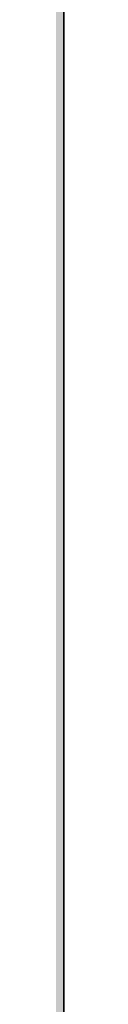
# Model space of a CAD drawing. Units: inches. Extents: x 2091 to 2899, y 967 to 2217.
# Tile 68 of 256: x 2212.144 to 2212.144, y 1101.165 to 1102.499. Entities that reach past the tile are written whole.
import ezdxf

# ---------------------------------------------------------------- set-up
doc = ezdxf.new("R2010")
doc.units = ezdxf.units.IN
doc.layers.add('A-WALL', color=7, linetype='Continuous', lineweight=35)
doc.layers.add('A-WALL-PATT', color=141, linetype='Continuous', lineweight=13, true_color=0xadddf7)

msp = doc.modelspace()

# ---------------------------------------------------------------- hatches: boundary and pattern name
at = {"layer": 'A-WALL-PATT'}
h = msp.add_hatch(color=256, dxfattribs=at)
h.dxf.hatch_style = 1
h.paths.add_polyline_path([(2212.1436, 1941.4191), (2387.6436, 1941.4191), (2387.6436, 1824.4191), (2392.1436, 1824.4191), (2392.1436, 1941.4191), (2609.6436, 1941.4191), (2609.6436, 1825.9191), (2614.1436, 1825.9191), (2614.1436, 1941.4191), (2794.1436, 1941.4191), (2794.1436, 1928.7622), (2803.1436, 1928.7622), (2803.1436, 2050.9191), (2203.1436, 2050.9191), (2203.1436, 1900.7579), (2212.1436, 1900.7579)])
h.paths.add_polyline_path([(2212.1436, 1945.9191), (2212.1436, 2041.9191), (2794.1436, 2041.9191), (2794.1436, 1945.9191), (2402.2482, 1945.9191), (2401.1024, 1945.7758), (2398.7024, 1945.7758)], flags=16)
h.paths.add_polyline_path([(2230.2299, 1948.0628), (2227.3499, 1949.5028), (2225.9099, 1951.9028), (2223.9899, 1952.8628), (2223.0299, 1955.2628), (2222.0699, 1959.5828), (2222.0699, 1963.4228), (2223.0299, 1965.6628), (2223.9899, 1965.3428), (2225.5859, 1963.8607), (2226.9115, 1964.9573), (2226.9489, 1965.9388), (2227.7783, 1966.9521), (2228.1999, 1968.8787), (2230.7099, 1964.8628), (2233.5899, 1966.3028), (2233.6073, 1966.3319), (2233.7727, 1964.9382), (2234.6338, 1963.6765), (2235.0299, 1963.9028), (2236.282, 1965.5724), (2235.9899, 1962.9428), (2237.9545, 1957.54), (2238.3899, 1957.9028), (2239.2159, 1960.3058), (2238.6546, 1966.385), (2238.6928, 1966.4381), (2238.8406, 1967.4997), (2238.7803, 1967.6875), (2238.8805, 1967.7868), (2238.6669, 1966.2518), (2239.2159, 1960.3058), (2238.3899, 1957.9028), (2236.9499, 1956.7028), (2234.5499, 1949.9828)], flags=0)
h.paths.add_polyline_path([(2278.012, 1948.0628), (2276.4964, 1947.8733), (2275.8498, 1947.6886), (2274.652, 1947.1028)], flags=0)
h.paths.add_polyline_path([(2269.852, 1955.7428), (2268.2762, 1956.6293), (2270.8673, 1956.3484), (2269.372, 1958.1428), (2268.715, 1959.1923), (2270.5698, 1958.7286), (2268.5807, 1961.9061), (2270.812, 1960.8919), (2270.812, 1963.4228), (2271.3933, 1964.7793), (2270.2918, 1966.1562), (2271.772, 1965.6628), (2272.1414, 1966.5248), (2273.9298, 1965.9286), (2275.6304, 1968.0543), (2276.3319, 1966.7219), (2276.5204, 1966.9521), (2276.942, 1968.8787), (2277.7343, 1967.6111), (2278.1399, 1969.4645), (2279.6591, 1967.0337), (2280.412, 1966.7828), (2280.9493, 1967.5888), (2281.6098, 1967.3686), (2282.1333, 1968.1538), (2282.3492, 1966.3334), (2282.3498, 1966.3326), (2283.4076, 1968.0954), (2283.7126, 1965.524), (2284.3202, 1964.6338), (2284.5118, 1964.8892), (2284.235, 1965.7048), (2284.5005, 1967.319), (2284.9079, 1965.4174), (2285.3963, 1966.0686), (2285.4328, 1966.2906), (2285.4733, 1966.1713), (2286.3539, 1967.3454), (2286.222, 1966.1582), (2287.6635, 1968.0802), (2287.714, 1968.4428), (2288.4816, 1969.0167), (2288.574, 1968.7289), (2288.9175, 1969.069), (2288.6068, 1966.8376), (2288.9287, 1963.3513), (2288.935, 1963.3568), (2288.9297, 1963.3404), (2289.0153, 1962.4139), (2290.1112, 1963.8751), (2290.1328, 1963.9426), (2290.2177, 1964.0171), (2290.1112, 1963.8751), (2289.1558, 1960.8916), (2288.594, 1959.2572), (2288.572, 1959.1028), (2289.532, 1960.5428), (2290.012, 1962.4628), (2290.1918, 1962.6427), (2289.7698, 1959.6886), (2286.8898, 1957.2886), (2284.4898, 1950.5686), (2283.3147, 1950.0463), (2283.292, 1949.9828), (2280.2901, 1948.6486), (2281.1298, 1948.6486), (2282.5698, 1948.1686), (2283.2047, 1948.0628), (2278.972, 1948.0628), (2276.092, 1949.5028), (2274.652, 1951.9028), (2272.732, 1952.8628)], flags=0)
h.paths.add_polyline_path([(2271.1589, 1958.0218), (2272.9698, 1955.8486), (2272.0098, 1960.1686), (2272.0098, 1964.0086), (2272.6244, 1965.4427), (2274.328, 1963.8607), (2275.6536, 1964.9573), (2275.6377, 1964.5391), (2277.4122, 1966.0069), (2277.033, 1965.1568), (2276.8299, 1964.9756), (2276.766, 1963.295), (2277.4496, 1962.6602), (2279.452, 1964.8628), (2282.332, 1966.3028), (2283.5298, 1966.8886), (2283.2945, 1966.7709), (2283.913, 1963.8847), (2284.8992, 1964.4483), (2284.732, 1962.9428), (2286.6966, 1957.54), (2287.132, 1957.9028), (2287.5419, 1959.0954), (2287.7794, 1958.4423), (2285.6827, 1956.6951), (2285.8765, 1959.7953), (2284.732, 1962.9428), (2284.8992, 1964.4483), (2283.913, 1963.8847), (2284.2238, 1962.4341), (2283.4244, 1963.6055), (2281.6098, 1962.5686), (2281.1298, 1960.1686), (2282.0898, 1956.3286), (2283.0498, 1952.9686), (2282.5698, 1950.5686), (2280.1698, 1948.6486), (2279.8833, 1948.7919), (2278.972, 1948.0628), (2278.972, 1949.0228), (2278.6723, 1949.3974), (2277.2898, 1950.0886), (2275.8498, 1952.4886), (2273.9298, 1953.4486), (2272.4898, 1954.8886), (2271.9216, 1954.8886), (2271.772, 1955.2628)], flags=0)
h.paths.add_polyline_path([(2311.9941, 1955.7428), (2312.0627, 1955.6742), (2312.0551, 1955.7085)], flags=0)
h.paths.add_polyline_path([(2331.9561, 1963.9518), (2333.3961, 1965.3918), (2331.0771, 1963.3568), (2330.9986, 1963.1115)], flags=0)
h.paths.add_polyline_path([(2310.5541, 1954.3028), (2307.0398, 1956.2799), (2310.7629, 1955.8763), (2312.4741, 1953.8228), (2313.4341, 1951.4228), (2315.3541, 1950.4628), (2316.7941, 1948.0628), (2317.4661, 1947.7268), (2319.3687, 1947.9646), (2317.7541, 1949.9828), (2317.5695, 1950.6105), (2316.7941, 1951.9028), (2314.8741, 1952.8628), (2313.9141, 1955.2628), (2311.5141, 1958.1428), (2309.3755, 1961.5592), (2311.5141, 1960.3371), (2311.5141, 1961.9828), (2310.6047, 1963.1196), (2311.7266, 1962.4785), (2312.4183, 1964.0926), (2312.256, 1964.2955), (2313.1941, 1963.9828), (2313.9141, 1965.6628), (2314.6468, 1965.4186), (2315.3541, 1966.3028), (2316.7941, 1967.7428), (2316.1574, 1966.9469), (2317.0341, 1965.2819), (2317.2226, 1965.5121), (2317.777, 1968.0458), (2318.4741, 1966.7219), (2318.6626, 1966.9521), (2319.0842, 1968.8787), (2321.207, 1965.4821), (2322.1614, 1966.9137), (2322.5541, 1966.7828), (2322.786, 1967.1306), (2322.8816, 1966.3243), (2323.312, 1965.7217), (2323.6513, 1965.8914), (2324.3965, 1967.1334), (2324.6569, 1964.9382), (2324.972, 1964.4766), (2325.3873, 1967.0015), (2325.9408, 1964.4183), (2327.2289, 1966.1358), (2327.1663, 1965.5724), (2328.0591, 1966.7628), (2328.2246, 1966.2475), (2329.668, 1967.6769), (2329.6646, 1967.6875), (2329.7648, 1967.7868), (2329.5511, 1966.2518), (2330.1001, 1960.3058), (2329.3328, 1958.0735), (2329.3131, 1957.9352), (2329.6341, 1958.2028), (2330.2341, 1959.1028), (2330.7141, 1961.0228), (2331.0341, 1961.3428), (2330.7141, 1959.1028), (2329.6341, 1958.2028), (2329.2741, 1957.6628), (2327.7121, 1956.3611), (2325.4341, 1949.9828), (2324.3338, 1949.4937), (2323.9941, 1948.5428), (2319.6741, 1946.6228), (2316.7941, 1948.0628), (2315.3541, 1950.4628), (2313.4341, 1951.4228)], flags=0)
h.paths.add_polyline_path([(2321.3357, 1947.952), (2321.1141, 1948.0628), (2321.1141, 1949.0228), (2319.1941, 1951.4228), (2316.7941, 1959.5828), (2316.6632, 1959.5828), (2315.3541, 1958.1428), (2314.3941, 1958.1428), (2313.1483, 1958.7091), (2312.9541, 1959.5828), (2312.9541, 1960.8919), (2315.8341, 1959.5828), (2316.6632, 1959.5828), (2317.3147, 1960.2994), (2315.0302, 1962.4207), (2316.3558, 1963.5173), (2316.3723, 1963.9516), (2316.4702, 1963.8607), (2317.7958, 1964.9573), (2317.7552, 1963.8897), (2319.1751, 1965.1568), (2319.4984, 1965.8814), (2321.1141, 1965.3428), (2323.2359, 1962.3724), (2325.6863, 1963.7726), (2325.5428, 1962.4806), (2325.1988, 1963.494), (2324.4785, 1963.0824), (2324.926, 1960.9941), (2324.0781, 1962.2365), (2322.4148, 1961.286), (2322.0741, 1959.5828), (2323.0341, 1955.7428), (2323.9941, 1952.3828), (2323.5141, 1949.9828), (2322.1427, 1948.8856), (2322.0741, 1948.5428)], flags=0)
h.paths.add_polyline_path([(2320.2075, 1963.3375), (2320.1541, 1963.4228), (2320.3941, 1963.5428)], flags=0)
h.paths.add_polyline_path([(2353.8505, 1965.8105), (2354.0305, 1965.7505), (2354.3305, 1966.4505), (2354.3305, 1966.9305)], flags=0)
h.paths.add_polyline_path([(2359.0206, 1969.0264), (2359.0984, 1968.9019), (2359.2335, 1969.5195), (2359.2335, 1969.9995)], flags=0)
h.paths.add_polyline_path([(2358.2567, 1966.6817), (2357.9836, 1966.348), (2358.2113, 1966.1462), (2358.4105, 1966.3896)], flags=0)
h.paths.add_polyline_path([(2357.7685, 1966.0588), (2357.7322, 1965.105), (2357.751, 1965.1206), (2357.7695, 1965.6065), (2357.7695, 1966.0578)], flags=0)
h.paths.add_polyline_path([(2359.1115, 1965.3045), (2359.1115, 1964.8245), (2359.8445, 1966.4675), (2359.8445, 1966.9475)], flags=0)
h.paths.add_polyline_path([(2360.2237, 1966.6214), (2360.6985, 1969.3625), (2360.6985, 1969.8425), (2360.2105, 1967.0255), (2360.2105, 1966.6425)], flags=0)
h.paths.add_polyline_path([(2363.4505, 1967.8905), (2363.4505, 1968.3705), (2362.4905, 1966.9305), (2362.656, 1966.6988)], flags=0)
h.paths.add_polyline_path([(2364.4755, 1966.0788), (2365.8505, 1968.3705), (2365.8505, 1968.8505), (2364.428, 1966.4796)], flags=0)
h.paths.add_polyline_path([(2366.3135, 1965.8525), (2366.3667, 1965.6958), (2366.8025, 1968.3455), (2366.8025, 1968.8255)], flags=0)
h.paths.add_polyline_path([(2367.1653, 1965.8035), (2367.2905, 1966.9305), (2367.2905, 1967.4105), (2367.1027, 1965.7201)], flags=0)
h.paths.add_polyline_path([(2370.0365, 1959.9735), (2371.0135, 1963.0245), (2371.0135, 1963.5045), (2370.0365, 1960.4535)], flags=0)
h.paths.add_polyline_path([(2371.6105, 1960.2105), (2372.5705, 1961.6505), (2372.5705, 1962.1305), (2371.8025, 1960.9785)], flags=0)
h.paths.add_polyline_path([(2350.8737, 1956.0051), (2351.9305, 1955.8905), (2354.4905, 1953.3305), (2353.8505, 1954.9305), (2351.4505, 1957.8105), (2347.9355, 1963.4255), (2347.9355, 1963.9055), (2351.4505, 1958.2905), (2353.7051, 1955.585), (2352.8905, 1959.2505), (2352.8905, 1959.7305), (2352.8905, 1961.9248), (2356.7305, 1959.7305), (2358.4545, 1961.6268), (2354.8105, 1965.0105), (2355.0309, 1965.2859), (2358.6911, 1961.8871), (2361.5305, 1965.0105), (2364.3765, 1966.4335), (2364.5244, 1965.1869), (2365.4545, 1963.8242), (2365.8811, 1964.068), (2365.3705, 1966.4505), (2365.3705, 1966.9305), (2366.8105, 1960.2105), (2366.8105, 1959.7305), (2366.3887, 1952.9814), (2367.7705, 1956.8505), (2368.6412, 1957.5761), (2366.8105, 1962.6105), (2366.8105, 1963.0905), (2368.7752, 1957.6877), (2369.2105, 1958.0505), (2370.0016, 1960.3519), (2369.4752, 1966.0527), (2369.5135, 1966.1058), (2369.5142, 1966.1109), (2369.4752, 1966.5327), (2369.5135, 1966.5858), (2369.6146, 1967.3126), (2369.1825, 1968.6585), (2369.1825, 1969.1385), (2369.601, 1967.8352), (2369.7012, 1967.9345), (2369.7179, 1968.0547), (2370.1452, 1968.3741), (2369.7787, 1968.0112), (2369.7012, 1967.4545), (2370.4682, 1968.214), (2369.6749, 1967.2658), (2369.5142, 1966.1109), (2370.0365, 1960.4535), (2370.0365, 1959.9735), (2369.4418, 1958.2432), (2370.6505, 1959.2505), (2371.0458, 1962.0176), (2371.1305, 1962.1305), (2370.6505, 1958.7705), (2367.7705, 1956.3705), (2365.3705, 1949.6505), (2362.0791, 1948.1876), (2363.4505, 1947.7305), (2361.0505, 1947.7305), (2360.0905, 1947.7305), (2357.1039, 1947.3572), (2360.0905, 1948.2105), (2358.1705, 1949.1705), (2356.7305, 1951.5705), (2354.8105, 1952.5305), (2351.9305, 1955.4105)], flags=0)
h.paths.add_polyline_path([(2361.0505, 1948.6905), (2359.1305, 1951.0905), (2356.7305, 1959.2505), (2355.7705, 1959.2505), (2352.8905, 1960.5596), (2352.8905, 1961.4448), (2355.8905, 1959.7305), (2356.7305, 1959.7305), (2356.8372, 1959.3678), (2361.5305, 1964.5305), (2363.2484, 1965.3894), (2364.9253, 1963.0418), (2362.4905, 1961.6505), (2362.0639, 1959.5172), (2362.9705, 1955.8905), (2363.9305, 1952.5305), (2363.9305, 1952.0505), (2363.4505, 1949.6505), (2361.0505, 1947.7305)], flags=0)
h.paths.add_polyline_path([(2359.1305, 1951.5705), (2359.2905, 1951.3705), (2361.0505, 1954.4505), (2361.0505, 1954.9305)], flags=0)
h.paths.add_polyline_path([(2357.2195, 1966.5455), (2356.7925, 1968.8145), (2356.7925, 1969.2945), (2357.2195, 1967.0255)], flags=0)
h.paths.add_polyline_path([(2361.0505, 1954.4505), (2361.5305, 1958.7705), (2361.5305, 1959.2505), (2361.0505, 1954.9305)], flags=0)
h.paths.add_polyline_path([(2402.5483, 1948.4861), (2402.3024, 1948.4158), (2402.5904, 1948.4158)], flags=0)
h.paths.add_polyline_path([(2394.1424, 1956.0958), (2395.6851, 1954.5532), (2396.7205, 1953.9707), (2396.0624, 1955.6158), (2395.2414, 1956.6011), (2395.8789, 1956.4417), (2395.1024, 1959.9358), (2395.1024, 1963.7758), (2396.0624, 1966.0158), (2397.0224, 1965.6958), (2398.6185, 1964.2138), (2399.9441, 1965.3103), (2399.9814, 1966.2918), (2400.8109, 1967.3052), (2401.2325, 1969.2317), (2403.5379, 1965.543), (2403.942, 1967.3893), (2404.7024, 1967.1358), (2405.4603, 1966.0748), (2406.6224, 1966.6558), (2406.6399, 1966.6849), (2406.8052, 1965.2912), (2406.9257, 1965.1147), (2407.3424, 1964.9758), (2407.8743, 1965.7737), (2408.1691, 1964.3981), (2409.3146, 1965.9254), (2409.2175, 1965.0511), (2409.4452, 1963.1312), (2410.3064, 1961.8695), (2410.7024, 1962.0958), (2411.4423, 1963.0823), (2411.1654, 1963.8978), (2411.6164, 1966.6398), (2411.7254, 1966.7911), (2411.8732, 1967.8527), (2411.8129, 1968.0405), (2411.9131, 1968.1398), (2411.6994, 1966.6048), (2412.2484, 1960.6588), (2413.2254, 1963.7098), (2414.3779, 1964.7212), (2414.5132, 1965.6927), (2414.4529, 1965.8805), (2414.5531, 1965.9798), (2414.3779, 1964.7212), (2414.5198, 1964.8457), (2414.3654, 1964.6311), (2414.3394, 1964.4448), (2414.8884, 1958.4988), (2414.0624, 1956.0958), (2412.6224, 1954.8958), (2410.1714, 1948.0329), (2410.0167, 1948.0844), (2405.9024, 1946.2558), (2405.9024, 1947.2158), (2405.2043, 1948.0886), (2404.2224, 1948.4158), (2403.2624, 1948.4158), (2400.3824, 1949.8558), (2399.6624, 1951.0558), (2397.9824, 1952.7358), (2397.0224, 1953.2158), (2395.6851, 1954.5532), (2392.6568, 1956.2569)], flags=0)
h.paths.add_polyline_path([(2409.0857, 1964.4074), (2409.1304, 1964.2757), (2409.2624, 1964.4958)], flags=0)
h.paths.add_polyline_path([(2397.7424, 1961.6158), (2398.7024, 1963.8558), (2399.6624, 1963.5358), (2401.4266, 1965.741), (2401.7914, 1966.5588), (2402.0714, 1965.0708), (2402.8355, 1964.3934), (2403.2624, 1964.9149), (2403.3381, 1964.7711), (2402.6155, 1963.9762), (2402.4986, 1960.9022), (2403.543, 1959.9325), (2404.4132, 1960.8897), (2404.7024, 1962.3358), (2407.9163, 1964.1724), (2409.5202, 1961.9269), (2410.9871, 1957.893), (2411.4224, 1958.2558), (2412.048, 1960.0756), (2412.4103, 1959.0791), (2411.6756, 1958.4668), (2411.6624, 1958.2558), (2411.6261, 1958.4255), (2409.9824, 1957.0558), (2407.5824, 1950.3358), (2403.2624, 1948.4158), (2403.2624, 1949.3758), (2401.3424, 1951.7758), (2399.4165, 1958.324), (2397.7424, 1959.0849), (2397.7424, 1959.9701), (2397.1024, 1960.3358), (2397.7424, 1960.0449)], flags=0)
h.paths.add_polyline_path([(2405.9024, 1952.9758), (2405.9504, 1953.4078), (2406.0167, 1953.1758)], flags=0)
h.paths.add_polyline_path([(2449.8178, 1967.114), (2449.7523, 1967.1358), (2449.7937, 1967.0779)], flags=0)
h.paths.add_polyline_path([(2451.6977, 1966.6181), (2451.7409, 1966.6901), (2451.6921, 1966.6657)], flags=0)
h.paths.add_polyline_path([(2454.3436, 1965.7376), (2455.7523, 1967.6158), (2455.9923, 1968.0958), (2454.3645, 1965.9254)], flags=0)
h.paths.add_polyline_path([(2457.5473, 1968.8638), (2457.7873, 1969.3438), (2457.0543, 1968.7958), (2457.0076, 1968.4603)], flags=0)
h.paths.add_polyline_path([(2456.9218, 1967.8567), (2456.8022, 1968.229), (2456.723, 1967.6598)], flags=0)
h.paths.add_polyline_path([(2457.3023, 1967.3768), (2457.5423, 1967.8568), (2456.8103, 1966.8398), (2456.7405, 1966.7002), (2456.749, 1966.6081)], flags=0)
h.paths.add_polyline_path([(2458.2753, 1963.7098), (2458.1553, 1963.3352), (2460.3543, 1965.2648), (2460.5943, 1965.7448)], flags=0)
h.paths.add_polyline_path([(2458.3923, 1962.8158), (2458.3641, 1962.6182), (2459.5923, 1964.2558), (2459.8323, 1964.7358)], flags=0)
h.paths.add_polyline_path([(2459.3523, 1962.8158), (2459.2723, 1962.4958), (2460.0723, 1963.2958), (2460.3123, 1963.7758)], flags=0)
h.paths.add_polyline_path([(2458.6803, 1960.6078), (2458.6323, 1960.4158), (2459.5923, 1961.8558), (2459.8323, 1962.3358)], flags=0)
h.paths.add_polyline_path([(2437.8382, 1956.2427), (2439.1923, 1956.0958), (2441.3523, 1953.9358), (2440.8723, 1955.1358), (2438.4723, 1958.0158), (2438.0716, 1958.656), (2438.7123, 1958.4958), (2440.6396, 1956.1831), (2439.9123, 1959.4558), (2439.9123, 1963.2958), (2441.3523, 1966.6558), (2441.5923, 1967.1358), (2441.1123, 1966.0158), (2442.0723, 1965.6958), (2443.989, 1968.0917), (2444.2413, 1966.7508), (2444.9168, 1966.1519), (2445.6766, 1967.0801), (2446.2553, 1969.7248), (2446.4953, 1970.2048), (2446.2824, 1969.2317), (2447.3627, 1967.5033), (2447.7203, 1969.5678), (2447.9603, 1970.0478), (2447.4855, 1967.3068), (2448.7923, 1965.2158), (2448.4723, 1964.8638), (2448.5523, 1964.7358), (2451.4521, 1966.1857), (2451.6151, 1964.8112), (2452.3079, 1963.7962), (2453.2345, 1964.3257), (2454.0723, 1960.4158), (2453.6287, 1953.3177), (2454.7923, 1956.5758), (2455.0323, 1957.0558), (2455.7188, 1957.6279), (2453.8323, 1962.8158), (2453.941, 1963.7936), (2453.3353, 1965.5778), (2453.8243, 1968.5508), (2454.0643, 1969.0308), (2453.5753, 1966.0578), (2454.0403, 1964.6879), (2453.8323, 1962.8158), (2455.7188, 1957.6279), (2456.3672, 1958.1682), (2457.0583, 1960.1788), (2457.2983, 1960.6588), (2456.4723, 1958.2558), (2457.7177, 1959.2937), (2457.6723, 1958.9758), (2454.89, 1956.6572), (2453.6141, 1953.0849), (2453.5923, 1952.7358), (2453.3523, 1952.2558), (2453.3596, 1952.3722), (2452.6323, 1950.3358), (2452.3923, 1949.8558), (2449.2038, 1948.4387), (2450.7123, 1947.9358), (2448.0723, 1947.9358), (2447.1123, 1947.9358), (2444.5523, 1947.6158), (2447.1996, 1948.3722), (2445.1923, 1949.3758), (2443.7523, 1951.7758), (2441.8323, 1952.7358), (2438.9523, 1955.6158)], flags=0)
h.paths.add_polyline_path([(2443.9923, 1959.9358), (2444.0403, 1959.7726), (2444.1216, 1959.862)], flags=0)
h.paths.add_polyline_path([(2442.9123, 1959.9358), (2443.0323, 1959.9358), (2442.4457, 1960.2025)], flags=0)
h.paths.add_polyline_path([(2444.9829, 1965.0197), (2445.2793, 1965.2648), (2445.5193, 1965.7448), (2444.994, 1965.3103)], flags=0)
h.paths.add_polyline_path([(2446.1333, 1965.0298), (2446.3304, 1965.4715), (2444.9703, 1964.2578), (2444.7303, 1963.7778)], flags=0)
h.paths.add_polyline_path([(2442.7923, 1959.4558), (2443.7523, 1959.4558), (2446.1523, 1951.2958), (2446.4123, 1951.7508), (2446.3923, 1951.7758), (2448.0806, 1954.7303), (2448.5523, 1958.9758), (2441.8323, 1965.2158), (2442.1549, 1965.6191), (2448.7923, 1959.4558), (2448.3123, 1955.1358), (2448.0723, 1954.6558), (2446.4123, 1951.7508), (2448.3123, 1949.3758), (2448.3123, 1948.4158), (2450.5409, 1950.1987), (2450.9523, 1952.2558), (2449.9923, 1955.6158), (2449.0323, 1959.4558), (2449.5123, 1961.8558), (2449.7523, 1962.3358), (2449.6749, 1961.9487), (2452.9945, 1963.8457), (2453.0644, 1963.5194), (2452.8846, 1963.7829), (2449.6749, 1961.9487), (2449.2723, 1959.9358), (2450.2323, 1956.0958), (2451.1923, 1952.7358), (2450.7123, 1950.3358), (2450.4723, 1949.8558), (2448.0723, 1947.9358), (2448.0723, 1948.5358), (2445.4323, 1949.8558), (2443.9923, 1952.2558), (2442.0723, 1953.2158), (2441.1123, 1955.6158), (2440.1523, 1959.9358), (2440.1523, 1960.6558)], flags=0)
h.paths.add_polyline_path([(2456.6923, 1966.9858), (2457.6083, 1968.0808), (2457.8483, 1968.5608), (2456.9323, 1967.4658)], flags=0)
h.paths.add_polyline_path([(2489.8966, 1966.5802), (2489.9429, 1966.1893), (2490.7475, 1967.5302), (2491.3191, 1968.9512)], flags=0)
h.paths.add_polyline_path([(2473.5625, 1956.4071), (2477.14, 1956.0193), (2476.9553, 1956.2408), (2475.108, 1957.2801), (2476.3475, 1956.9702), (2475.1869, 1958.8242), (2476.9191, 1958.3912), (2475.4116, 1960.7993), (2477.7875, 1959.7193), (2477.7875, 1962.2502), (2477.6374, 1962.4379), (2477.8226, 1962.3321), (2478.3591, 1963.5841), (2478.3591, 1963.6712), (2477.3243, 1964.9646), (2478.7148, 1964.5011), (2479.3191, 1965.9112), (2480.2791, 1965.5912), (2481.784, 1967.4722), (2482.1165, 1965.7052), (2482.8806, 1965.0278), (2483.2093, 1965.4294), (2483.2202, 1965.7151), (2483.0759, 1965.989), (2483.7118, 1966.7658), (2484.1305, 1968.6792), (2484.7021, 1970.1002), (2484.4892, 1969.1271), (2486.5029, 1965.9051), (2487.3875, 1965.6102), (2488.1534, 1966.7591), (2488.717, 1965.9701), (2489.2001, 1966.2116), (2489.3307, 1965.111), (2490.3939, 1963.6225), (2490.6608, 1963.775), (2490.4939, 1964.5536), (2490.9231, 1963.9248), (2491.3191, 1964.1512), (2491.3334, 1964.1702), (2491.2105, 1964.5322), (2491.2818, 1964.9655), (2491.4258, 1964.2934), (2494.0765, 1967.8276), (2494.4979, 1966.5149), (2494.5982, 1966.6142), (2494.6895, 1967.2702), (2495.1067, 1967.5822), (2495.1298, 1967.7481), (2495.0696, 1967.9359), (2495.1698, 1968.0351), (2495.0318, 1967.0436), (2495.7538, 1967.7587), (2494.9821, 1966.6864), (2494.9561, 1966.5002), (2495.479, 1960.8369), (2495.9105, 1962.1842), (2496.4821, 1963.6052), (2496.0727, 1962.3266), (2496.7689, 1962.9375), (2496.5991, 1962.7112), (2496.1191, 1959.3512), (2496.7329, 1960.2718), (2496.9875, 1961.2902), (2497.5591, 1962.7112), (2497.0791, 1960.7912), (2496.5075, 1959.3702), (2495.5475, 1957.9302), (2492.7588, 1955.6064), (2490.8391, 1950.2312), (2490.2675, 1948.8102), (2485.9475, 1946.8902), (2483.0675, 1948.3302), (2481.6275, 1950.7302), (2479.7075, 1951.6902), (2476.8275, 1954.5702)], flags=0)
h.paths.add_polyline_path([(2485.577, 1948.3134), (2485.5591, 1948.3112), (2485.5788, 1948.3112)], flags=0)
h.paths.add_polyline_path([(2478.6451, 1954.5512), (2478.109, 1956.9633), (2479.3191, 1955.5112), (2480.2791, 1953.1112), (2482.1991, 1952.1512), (2483.6391, 1949.7512), (2486.5191, 1948.3112), (2486.5191, 1949.2712), (2484.7393, 1951.4959), (2484.0275, 1950.2502), (2481.6275, 1958.4102), (2482.3751, 1959.2327), (2482.1991, 1959.8312), (2483.1976, 1960.9295), (2479.7075, 1964.1702), (2480.6034, 1965.2901), (2481.8752, 1964.1091), (2482.6664, 1964.7636), (2482.6154, 1963.4218), (2482.9892, 1963.0747), (2484.0085, 1963.9842), (2484.6836, 1965.4975), (2484.5801, 1965.4052), (2485.3573, 1967.1471), (2485.1206, 1965.7812), (2486.4275, 1963.6902), (2488.1454, 1964.5492), (2489.8223, 1962.2016), (2490.7475, 1962.7302), (2491.9997, 1964.3998), (2492.076, 1965.0873), (2492.2129, 1964.6841), (2492.4854, 1965.0474), (2492.2791, 1963.1912), (2494.2438, 1957.7884), (2494.5625, 1958.054), (2494.9335, 1959.1332), (2495.5051, 1960.5542), (2494.6791, 1958.1512), (2494.1075, 1956.7302), (2494.5625, 1958.054), (2493.4085, 1957.0923), (2491.7075, 1961.7702), (2491.9997, 1964.3998), (2490.7475, 1962.7302), (2487.712, 1960.9957), (2487.4791, 1959.8312), (2488.4391, 1955.9912), (2489.3991, 1952.6312), (2488.9191, 1950.2312), (2488.5769, 1949.9574), (2488.3475, 1948.8102), (2487.6517, 1948.2536), (2487.4791, 1948.3112), (2486.5191, 1948.3112), (2483.6391, 1949.7512), (2482.1991, 1952.1512), (2480.2791, 1953.1112), (2478.8391, 1954.5512)], flags=0)
h.paths.add_polyline_path([(2526.6483, 1966.9875), (2526.5173, 1967.0312), (2526.6001, 1966.9153)], flags=0)
h.paths.add_polyline_path([(2528.4706, 1966.4467), (2528.5745, 1966.6197), (2528.4571, 1966.561)], flags=0)
h.paths.add_polyline_path([(2534.1333, 1967.4962), (2534.1567, 1967.5428), (2534.0598, 1967.4083)], flags=0)
h.paths.add_polyline_path([(2536.1619, 1964.0506), (2535.1573, 1962.7112), (2535.1009, 1962.3159), (2536.1173, 1963.6712), (2536.4205, 1964.2775)], flags=0)
h.paths.add_polyline_path([(2535.1573, 1959.8312), (2536.1173, 1961.2712), (2536.5973, 1962.2312), (2535.2533, 1960.2152)], flags=0)
h.paths.add_polyline_path([(2513.249, 1956.2848), (2516.2212, 1955.9626), (2514.9973, 1957.4312), (2514.1958, 1958.7115), (2515.4773, 1958.3912), (2516.9319, 1956.6457), (2516.4373, 1958.8712), (2516.4373, 1962.7112), (2516.8727, 1963.727), (2515.3464, 1965.6348), (2517.3973, 1964.9512), (2517.8773, 1966.0712), (2518.3573, 1967.0312), (2517.8773, 1965.9112), (2518.8373, 1965.5912), (2520.4866, 1967.6527), (2520.7663, 1966.1662), (2521.5304, 1965.4887), (2521.7814, 1965.7954), (2521.8009, 1966.3073), (2521.4778, 1966.9209), (2521.2463, 1967.1262), (2521.1777, 1967.4909), (2521.4778, 1966.9209), (2522.0104, 1966.4487), (2522.2574, 1966.7504), (2522.7803, 1969.1402), (2523.2603, 1970.1002), (2523.0474, 1969.1271), (2524.6731, 1966.5259), (2526.0373, 1966.0712), (2526.7952, 1965.0101), (2527.9771, 1965.601), (2528.1401, 1964.2266), (2528.6646, 1963.4582), (2529.3886, 1963.8719), (2529.3297, 1964.147), (2529.4813, 1963.9248), (2529.8773, 1964.1512), (2529.984, 1964.2934), (2529.7891, 1965.2032), (2530.0624, 1964.3979), (2532.8025, 1968.0513), (2533.1478, 1966.9759), (2533.248, 1967.0751), (2533.3393, 1967.7312), (2533.6728, 1967.9805), (2533.728, 1968.0351), (2533.5143, 1966.5002), (2534.0247, 1960.9725), (2534.5603, 1962.6452), (2535.0403, 1963.6052), (2534.0633, 1960.5542), (2533.2373, 1958.1512), (2534.2882, 1959.0268), (2534.1973, 1958.3912), (2531.5126, 1956.1539), (2529.3973, 1950.2312), (2528.9173, 1949.2712), (2526.4488, 1948.174), (2527.4773, 1947.8312), (2530.3573, 1947.3512), (2524.5973, 1947.3512), (2521.7173, 1948.7912), (2520.2773, 1951.1912), (2518.3573, 1952.1512), (2515.4773, 1955.0312)], flags=0)
h.paths.add_polyline_path([(2523.9348, 1967.1903), (2523.6195, 1966.4837), (2523.7705, 1966.2421)], flags=0)
h.paths.add_polyline_path([(2518.8373, 1953.1112), (2517.8773, 1955.5112), (2516.885, 1959.9768), (2516.9173, 1959.9621), (2516.9173, 1962.0254), (2520.7573, 1959.8312), (2522.0249, 1961.2255), (2518.3573, 1964.6312), (2519.0026, 1965.4377), (2520.4334, 1964.1091), (2521.3011, 1964.8269), (2521.2452, 1963.3553), (2525.6383, 1959.276), (2526.0373, 1961.2712), (2529.3973, 1963.1912), (2530.6495, 1964.8607), (2530.6647, 1964.9976), (2530.692, 1964.9173), (2531.0878, 1965.4451), (2530.946, 1964.1689), (2530.692, 1964.9173), (2529.3973, 1963.1912), (2526.3625, 1961.457), (2526.0373, 1959.8312), (2526.9973, 1955.9912), (2527.9573, 1952.6312), (2527.4773, 1950.2312), (2527.1345, 1949.9569), (2526.9739, 1949.1541), (2526.6973, 1949.0312), (2524.5973, 1947.3512), (2524.5973, 1948.3112), (2524.2773, 1948.7112), (2522.1973, 1949.7512), (2520.7573, 1952.1512)], flags=0)
h.paths.add_polyline_path([(2520.2773, 1958.8712), (2520.8533, 1959.5048), (2523.1573, 1951.6712), (2524.6139, 1954.2201), (2524.5973, 1954.0712), (2522.6773, 1950.7112)], flags=0)
h.paths.add_polyline_path([(2559.3709, 1966.3112), (2559.3984, 1966.3249), (2559.4019, 1966.3453)], flags=0)
h.paths.add_polyline_path([(2549.7709, 1957.1912), (2552.6509, 1954.3112), (2552.134, 1955.6035), (2550.6109, 1957.4312), (2547.0959, 1963.0462), (2545.7759, 1965.2062), (2549.2909, 1959.5912), (2551.6909, 1956.7112), (2550.7929, 1960.7521), (2550.7309, 1960.7803), (2550.7309, 1964.8712), (2551.6909, 1967.1112), (2552.6509, 1966.7912), (2554.247, 1965.3091), (2555.0343, 1965.9603), (2555.5817, 1966.6446), (2555.6099, 1967.3872), (2556.4394, 1968.4005), (2556.861, 1970.3271), (2559.3709, 1966.3112), (2560.6909, 1964.1512), (2562.4088, 1965.0101), (2561.6509, 1966.0712), (2560.3309, 1968.2312), (2561.7585, 1966.2325), (2562.3472, 1967.1156), (2562.4337, 1966.3866), (2563.1278, 1965.3696), (2563.5709, 1965.5912), (2563.5884, 1965.6202), (2563.3625, 1967.5235), (2563.7225, 1965.8438), (2565.06, 1968.073), (2564.7329, 1965.1287), (2565.1176, 1963.3334), (2567.4446, 1966.4361), (2567.3156, 1967.8333), (2567.3538, 1967.8864), (2567.5016, 1968.9481), (2567.4413, 1969.1359), (2567.5416, 1969.2351), (2567.3279, 1967.7002), (2567.8769, 1961.7542), (2568.7467, 1964.4703), (2568.6356, 1965.6733), (2568.6738, 1965.7264), (2568.8216, 1966.7881), (2568.7613, 1966.9759), (2568.8616, 1967.0751), (2568.6479, 1965.5402), (2568.7261, 1964.693), (2568.8539, 1964.8052), (2568.7467, 1964.4703), (2568.8172, 1963.7063), (2568.9709, 1963.9112), (2568.8661, 1963.1773), (2569.1969, 1959.5942), (2568.3709, 1957.1912), (2566.9309, 1955.9912), (2564.6203, 1949.5214), (2564.6509, 1949.5112), (2564.6166, 1949.5112), (2564.5309, 1949.2712), (2560.2109, 1947.3512), (2557.3309, 1948.7912), (2556.0452, 1950.934), (2556.0109, 1950.9512), (2555.8566, 1951.2083), (2553.9709, 1952.1512), (2551.0909, 1955.0312), (2546.6501, 1957.5295)], flags=0)
h.paths.add_polyline_path([(2567.0258, 1959.3302), (2567.035, 1959.3049), (2567.0509, 1959.3512)], flags=0)
h.paths.add_polyline_path([(2551.9683, 1962.5184), (2553.0109, 1964.9512), (2553.9709, 1964.6312), (2555.567, 1963.1491), (2556.8926, 1964.2456), (2556.9299, 1965.2272), (2557.144, 1965.4887), (2556.4201, 1966.1306), (2556.3914, 1966.105), (2556.3799, 1966.1662), (2556.4201, 1966.1306), (2556.9519, 1966.6052), (2557.0921, 1966.9195), (2557.5709, 1966.0102), (2557.7594, 1966.2405), (2557.4179, 1964.6802), (2556.8926, 1964.2456), (2556.8071, 1961.9976), (2560.6909, 1958.3912), (2560.6355, 1957.8927), (2560.8109, 1957.1912), (2561.7709, 1953.8312), (2561.2909, 1951.4312), (2559.1104, 1949.6868), (2559.1565, 1949.6292), (2563.0265, 1951.3492), (2562.6109, 1949.2712), (2560.2109, 1947.3512), (2560.2109, 1948.3112), (2559.2509, 1949.5112), (2558.8909, 1949.5112), (2558.8909, 1949.9612), (2558.2909, 1950.7112), (2558.0537, 1951.5177), (2556.9709, 1952.8712), (2555.0679, 1959.3415), (2552.0509, 1961.0654), (2552.0509, 1962.4712)], flags=0)
h.paths.add_polyline_path([(2588.33, 1958.3912), (2588.6102, 1958.111), (2588.5534, 1958.3669)], flags=0)
h.paths.add_polyline_path([(2594.7455, 1950.4931), (2593.9575, 1953.172), (2593.13, 1954.5512), (2591.21, 1955.5112), (2590.25, 1957.9112), (2588.309, 1960.2404), (2586.1773, 1961.2093), (2587.85, 1960.7912), (2587.2534, 1961.7442), (2588.4413, 1961.0654), (2588.4413, 1962.6555), (2588.4217, 1962.6653), (2588.4413, 1962.7112), (2586.914, 1964.6203), (2588.8771, 1963.728), (2589.29, 1964.6915), (2589.29, 1966.0712), (2590.25, 1968.3112), (2591.21, 1967.9912), (2592.8061, 1966.5091), (2594.1317, 1967.6056), (2594.169, 1968.5872), (2594.9985, 1969.6005), (2595.4201, 1971.5271), (2597.93, 1967.5112), (2600.81, 1968.9512), (2600.8275, 1968.9802), (2600.9928, 1967.5866), (2601.854, 1966.3248), (2602.1071, 1966.4695), (2602.2364, 1967.2551), (2602.3567, 1966.6934), (2603.5022, 1968.2207), (2603.21, 1965.5912), (2605.1747, 1960.1884), (2605.5069, 1960.4652), (2605.026, 1965.6733), (2605.0642, 1965.7264), (2605.212, 1966.7881), (2605.1517, 1966.9759), (2605.252, 1967.0751), (2605.3433, 1967.7312), (2605.9529, 1968.1869), (2605.8748, 1969.0333), (2605.913, 1969.0864), (2606.0608, 1970.1481), (2606.0005, 1970.3359), (2606.1007, 1970.4351), (2605.887, 1968.9002), (2606.436, 1962.9542), (2605.61, 1960.5512), (2605.997, 1960.8737), (2606.5643, 1962.6452), (2608.2415, 1964.1169), (2608.01, 1963.1912), (2607.05, 1961.7512), (2606.6315, 1961.4024), (2606.2013, 1958.3912), (2603.3213, 1955.9912), (2600.9213, 1949.2712), (2596.6013, 1947.3512), (2593.7213, 1948.7912), (2592.8573, 1950.2312), (2592.65, 1950.2312)], flags=0)
h.paths.add_polyline_path([(2596.6013, 1947.3512), (2596.6013, 1948.3112), (2594.6813, 1950.7112), (2596.155, 1953.29), (2595.53, 1954.0712), (2593.1992, 1961.996), (2592.6513, 1962.5047), (2591.7802, 1963.0025), (2593.283, 1964.2456), (2593.3203, 1965.2272), (2594.1498, 1966.2405), (2594.5714, 1968.1671), (2596.1827, 1965.589), (2596.9513, 1966.4345), (2598.0413, 1966.0712), (2598.7992, 1965.0101), (2599.9613, 1965.5912), (2599.9788, 1965.6202), (2600.1441, 1964.2266), (2601.0053, 1962.9648), (2601.4013, 1963.1912), (2602.6535, 1964.8607), (2602.3613, 1962.2312), (2603.7927, 1958.2947), (2601.9776, 1953.2124), (2601.9462, 1952.7095), (2599.4688, 1951.6084), (2599.0013, 1949.2712)], flags=0)
h.paths.add_polyline_path([(2597.5613, 1958.8712), (2597.671, 1959.4194), (2597.5951, 1958.7362)], flags=0)
h.paths.add_polyline_path([(2623.6663, 1961.2544), (2625.5192, 1960.7912), (2624.9655, 1961.6755), (2627.1992, 1960.6603), (2627.1992, 1961.1512), (2626.9592, 1962.2312), (2626.9592, 1963.4912), (2625.5823, 1965.2122), (2626.9592, 1964.4254), (2626.9592, 1965.8312), (2626.8692, 1965.8612), (2627.9192, 1968.3112), (2628.8792, 1967.9912), (2630.4752, 1966.5091), (2631.8008, 1967.6056), (2631.8382, 1968.5872), (2632.6676, 1969.6005), (2633.0892, 1971.5271), (2635.5992, 1967.5112), (2638.4792, 1968.9512), (2638.4966, 1968.9802), (2638.662, 1967.5866), (2639.1763, 1966.833), (2639.7802, 1967.8396), (2640.0258, 1966.6934), (2641.1713, 1968.2207), (2640.8792, 1965.5912), (2641.1143, 1964.9446), (2641.4113, 1965.3407), (2641.3081, 1964.4116), (2642.8438, 1960.1884), (2643.2792, 1960.5512), (2644.0847, 1962.8947), (2643.7839, 1966.1533), (2643.8068, 1966.1852), (2643.6007, 1968.4181), (2643.5228, 1968.6606), (2643.7299, 1970.1481), (2643.6696, 1970.3359), (2643.7698, 1970.4351), (2643.5562, 1968.9002), (2643.6007, 1968.4181), (2643.9096, 1967.4559), (2644.0098, 1967.5551), (2643.8117, 1966.1321), (2644.1052, 1962.9542), (2644.2388, 1961.3508), (2644.7192, 1961.7512), (2645.0329, 1962.2217), (2645.3222, 1963.1252), (2646.0764, 1963.787), (2645.0329, 1962.2217), (2644.3452, 1960.0742), (2643.5192, 1957.6712), (2642.0792, 1956.4712), (2639.7196, 1949.8644), (2639.8755, 1949.8384), (2635.3592, 1947.8312), (2632.4792, 1949.2712), (2631.0392, 1951.6712), (2629.1192, 1952.6312), (2628.1592, 1955.0312), (2625.7592, 1957.9112)], flags=0)
h.paths.add_polyline_path([(2627.8163, 1956.574), (2627.3737, 1958.5657), (2626.3763, 1959.7626), (2627.1992, 1959.3512), (2627.3737, 1958.5657), (2627.9192, 1957.9112), (2628.8792, 1955.5112), (2630.7992, 1954.5512), (2632.2392, 1952.1512), (2633.315, 1951.6132), (2631.0392, 1959.3512), (2631.4978, 1959.8557), (2630.7992, 1962.2312), (2631.4499, 1962.9469), (2630.7152, 1963.6291), (2632.0408, 1964.7256), (2632.0782, 1965.7072), (2632.2922, 1965.9687), (2631.7053, 1966.4891), (2633.1364, 1967.7661), (2633.3292, 1968.6471), (2634.6747, 1966.4943), (2635.2085, 1967.0814), (2636.7992, 1966.5512), (2637.6764, 1967.867), (2638.9939, 1966.0225), (2639.7053, 1966.429), (2641.1192, 1959.8312), (2640.9301, 1956.8057), (2639.4392, 1952.6312), (2638.2275, 1952.0926), (2637.7592, 1949.7512), (2635.3592, 1947.8312), (2635.3592, 1948.7912), (2633.4392, 1951.1912), (2633.315, 1951.6132), (2632.2392, 1952.1512), (2630.7992, 1954.5512), (2628.8792, 1955.5112)], flags=0)
h.paths.add_polyline_path([(2637.7592, 1953.8312), (2637.2792, 1955.5112), (2636.3192, 1959.3512), (2636.7992, 1961.7512), (2639.2339, 1963.1425), (2637.5571, 1965.4901), (2638.7389, 1966.081), (2638.902, 1964.7066), (2639.7631, 1963.4448), (2636.7992, 1961.7512), (2636.5325, 1960.4178), (2637.0392, 1958.3912), (2637.9992, 1955.0312)], flags=0)
h.paths.add_polyline_path([(2668.5674, 1951.4312), (2667.6074, 1953.8312), (2665.2074, 1956.7112), (2662.2939, 1961.3653), (2665.4474, 1959.5912), (2666.6474, 1958.3912), (2666.6474, 1959.9752), (2666.0583, 1960.6821), (2666.6474, 1960.3454), (2666.6474, 1961.9912), (2666.7001, 1962.1141), (2666.4074, 1963.4312), (2666.4074, 1967.2712), (2667.3674, 1969.5112), (2668.3274, 1969.1912), (2669.9235, 1967.7091), (2671.2491, 1968.8056), (2671.2864, 1969.7872), (2672.1159, 1970.8005), (2672.5375, 1972.7271), (2675.0474, 1968.7112), (2677.9274, 1970.1512), (2677.9449, 1970.1802), (2678.1102, 1968.7866), (2678.9713, 1967.5248), (2679.3674, 1967.7512), (2680.6196, 1969.4207), (2680.3274, 1966.7912), (2682.2921, 1961.3884), (2682.7274, 1961.7512), (2683.3583, 1963.5866), (2683.2321, 1964.9533), (2683.2703, 1965.0064), (2683.3932, 1965.8891), (2683.36, 1966.2492), (2683.3578, 1966.2559), (2683.3592, 1966.2572), (2682.9921, 1970.2333), (2683.0303, 1970.2864), (2683.1781, 1971.3481), (2683.1178, 1971.5359), (2683.2181, 1971.6351), (2683.0044, 1970.1002), (2683.3592, 1966.2572), (2683.4581, 1966.3551), (2683.3932, 1965.8891), (2683.4139, 1965.665), (2684.4238, 1966.8723), (2683.5534, 1964.1542), (2683.3583, 1963.5866), (2683.7934, 1958.8742), (2682.9674, 1956.4712), (2681.5274, 1955.2712), (2680.1092, 1951.3003), (2680.0849, 1950.9116), (2679.9768, 1950.9296), (2679.1274, 1948.5512), (2674.8074, 1946.6312), (2671.9274, 1948.0712), (2670.4874, 1950.4712)], flags=0)
h.paths.add_polyline_path([(2671.9357, 1953.227), (2671.6874, 1953.3512), (2670.2474, 1955.7512), (2668.3274, 1956.7112), (2667.3567, 1959.1378), (2669.5274, 1958.1512), (2670.4874, 1958.1512), (2671.4794, 1959.2424), (2670.6844, 1961.9454), (2668.8896, 1963.612), (2667.3074, 1964.3312), (2668.5674, 1963.9112), (2668.8309, 1964.2406), (2670.2474, 1963.4312), (2672.4221, 1965.8234), (2672.7775, 1967.4471), (2673.2341, 1966.7165), (2674.4119, 1968.0121), (2673.9806, 1965.5221), (2675.2874, 1963.4312), (2675.5541, 1963.5645), (2675.9324, 1965.4562), (2676.2474, 1965.3512), (2677.0053, 1964.2901), (2678.1674, 1964.8712), (2679.6074, 1967.2712), (2680.3274, 1963.9112), (2680.3066, 1963.5775), (2680.3472, 1963.4576), (2680.8596, 1964.1407), (2680.5674, 1961.5112), (2681.1036, 1960.0366), (2678.8874, 1953.8312), (2677.0925, 1953.0334), (2677.6874, 1950.9512), (2677.2074, 1948.5512), (2674.8074, 1946.6312), (2674.8074, 1947.5912), (2672.8874, 1949.9912)], flags=0)
h.paths.add_polyline_path([(2673.9846, 1951.9112), (2674.5674, 1952.9312), (2674.5674, 1951.9112), (2676.9674, 1953.8312), (2677.4474, 1956.2312), (2676.4874, 1959.5912), (2676.2474, 1960.5512), (2679.7296, 1962.541), (2680.0593, 1961.0025), (2679.2113, 1962.2448), (2676.2474, 1960.5512), (2676.4874, 1959.5912), (2677.4474, 1956.2312), (2676.9674, 1953.8312), (2674.5674, 1951.9112)], flags=0)
h.paths.add_polyline_path([(2707.4793, 1952.8147), (2706.5193, 1955.2147), (2705.5593, 1959.5347), (2705.5593, 1963.3747), (2706.5193, 1965.6147), (2707.4793, 1965.2947), (2709.0753, 1963.8126), (2710.401, 1964.9091), (2710.4383, 1965.8907), (2711.2677, 1966.904), (2711.6893, 1968.8306), (2714.1993, 1964.8147), (2717.0793, 1966.2547), (2717.0967, 1966.2837), (2717.2621, 1964.8901), (2718.1232, 1963.6283), (2718.5193, 1963.8547), (2719.7715, 1965.5242), (2719.4793, 1962.8947), (2721.4439, 1957.4919), (2721.8793, 1957.8547), (2722.7053, 1960.2577), (2722.144, 1966.3368), (2722.1822, 1966.3899), (2722.33, 1967.4516), (2722.2697, 1967.6393), (2722.37, 1967.7386), (2722.1563, 1966.2037), (2722.7053, 1960.2577), (2721.8793, 1957.8547), (2720.4393, 1956.6547), (2718.0393, 1949.9347), (2713.7193, 1948.0147), (2710.8393, 1949.4547), (2709.3993, 1951.8547)], flags=0)
h.paths.add_polyline_path([(2749.3012, 1952.8147), (2748.3412, 1955.2147), (2747.3812, 1959.5347), (2747.3812, 1963.3747), (2748.3412, 1965.6147), (2749.3012, 1965.2947), (2750.8973, 1963.8126), (2752.2229, 1964.9091), (2752.2602, 1965.8907), (2753.0897, 1966.904), (2753.5113, 1968.8306), (2756.0212, 1964.8147), (2758.9012, 1966.2547), (2758.9187, 1966.2837), (2759.084, 1964.8901), (2759.9452, 1963.6283), (2760.3412, 1963.8547), (2761.5934, 1965.5242), (2761.3012, 1962.8947), (2763.2659, 1957.4919), (2763.7012, 1957.8547), (2764.5272, 1960.2577), (2763.9659, 1966.3368), (2764.0042, 1966.3899), (2764.1519, 1967.4516), (2764.0917, 1967.6393), (2764.1919, 1967.7386), (2763.9782, 1966.2037), (2764.5272, 1960.2577), (2763.7012, 1957.8547), (2762.2612, 1956.6547), (2759.8612, 1949.9347), (2755.5412, 1948.0147), (2752.6612, 1949.4547), (2751.2212, 1951.8547)], flags=0)
h.paths.add_polyline_path([(2212.1436, 1819.9345), (2203.1436, 1819.9345), (2203.1436, 1739.9795), (2212.1436, 1739.9795), (2212.1436, 1780.9191), (2392.1436, 1780.9191), (2392.1436, 1783.9191), (2212.1436, 1783.9191)])
h.paths.add_polyline_path([(2803.1436, 1847.9388), (2794.1436, 1847.9388), (2794.1436, 1785.4191), (2609.6436, 1785.4191), (2493.8756, 1785.4191), (2493.8756, 1780.9191), (2609.6436, 1780.9191), (2794.1436, 1780.9191), (2794.1436, 1696.9191), (2609.3756, 1696.9191), (2609.3756, 1742.9191), (2604.8756, 1742.9191), (2604.8756, 1644.4191), (2609.3756, 1644.4191), (2609.3756, 1692.4191), (2794.1436, 1692.4191), (2794.1436, 1668.1647), (2803.1436, 1668.1647)])
h.paths.add_polyline_path([(2392.1436, 1740.4191), (2387.6436, 1740.4191), (2387.6436, 1629.4191), (2212.1436, 1629.4191), (2212.1436, 1659.1562), (2203.1436, 1659.1562), (2203.1436, 1494.0894), (2212.1436, 1494.0894), (2212.1436, 1627.9191), (2392.1436, 1627.9191)])
h.paths.add_polyline_path([(2457.8756, 1780.9191), (2453.3756, 1780.9191), (2453.3756, 1644.4191), (2568.8756, 1644.4191), (2568.8756, 1648.9191), (2457.8756, 1648.9191)])
h.paths.add_polyline_path([(2545.1436, 1591.9191), (2540.6436, 1591.9191), (2540.6436, 1567.9191), (2468.6436, 1567.9191), (2468.6436, 1627.9191), (2509.1436, 1627.9191), (2509.1436, 1632.4191), (2464.1436, 1632.4191), (2464.1436, 1563.4191), (2545.1436, 1563.4191)])
h.paths.add_polyline_path([(2268.6436, 1555.9191), (2212.1436, 1555.9191), (2212.1436, 1551.4191), (2268.6436, 1551.4191)], flags=17)
h.paths.add_polyline_path([(2212.1436, 1413.2661), (2203.1436, 1413.2661), (2203.1436, 1233.0704), (2212.1436, 1233.0704)])
h.paths.add_polyline_path([(2267.6436, 1351.9191), (2212.1436, 1351.9191), (2212.1436, 1347.4191), (2267.6436, 1347.4191)], flags=17)
h.paths.add_polyline_path([(2456.6436, 1489.4191), (2452.1436, 1489.4191), (2452.1436, 1351.9191), (2312.6436, 1351.9191), (2312.6436, 1347.4191), (2456.6436, 1347.4191)])
h.paths.add_polyline_path([(2472.3702, 1455.4191), (2467.8702, 1455.4191), (2467.8702, 1347.4191), (2472.3702, 1347.4191)])
h.paths.add_polyline_path([(2794.1436, 1351.9191), (2543.3702, 1351.9191), (2543.3702, 1347.4191), (2794.1436, 1347.4191)], flags=17)
h.paths.add_polyline_path([(2312.6436, 1347.4191), (2308.1436, 1347.4191), (2308.1436, 1302.1618), (2308.342, 1302.1643), (2308.1436, 1298.1692), (2308.1436, 1275.4191), (2212.1436, 1275.4191), (2212.1436, 1270.9191), (2312.6436, 1270.9191)], flags=17)
h.paths.add_polyline_path([(2212.1436, 1152.2471), (2203.1436, 1152.2471), (2203.1436, 1090.9191), (2803.1436, 1090.9191), (2803.1436, 1392.7136), (2794.1436, 1392.7136), (2794.1436, 1143.4191), (2548.0324, 1143.4191), (2548.0324, 1138.9191), (2794.1436, 1138.9191), (2794.1436, 1099.9191), (2212.1436, 1099.9191)])
h.paths.add_polyline_path([(2471.5324, 1266.3285, 0.031658), (2467.0324, 1269.9458), (2467.0324, 1143.4191), (2471.5324, 1143.4191), (2471.5324, 1148.8191)], flags=17)
h.paths.add_polyline_path([(2803.1436, 1587.3414), (2794.1436, 1587.3414), (2794.1436, 1473.5369), (2803.1436, 1473.5369)])
h.paths.add_polyline_path([(2794.1436, 1536.4191), (2651.1436, 1536.4191), (2651.1436, 1531.9191), (2794.1436, 1531.9191)])
h.paths.add_polyline_path([(2614.1436, 1620.4191), (2609.6436, 1620.4191), (2609.6436, 1536.4191), (2614.1436, 1536.4191)])
h.paths.add_polyline_path([(2271.0827, 1964.3172), (2776.853, 1964.3172), (2776.853, 2037.1696), (2271.0827, 2037.1696)], flags=8)
h.paths.add_polyline_path([(2380.6493, 1536.8241), (2461.0408, 1536.8241), (2461.0408, 1554.6526), (2380.6493, 1554.6526)], flags=9)
h.paths.add_polyline_path([(2203.655, 1608.8153), (2316.1184, 1608.8153), (2316.1184, 1621.9184), (2203.655, 1621.9184)], flags=24)
h.paths.add_polyline_path([(2212.6773, 1313.5041), (2282.5915, 1313.5041), (2282.5915, 1322.7452), (2212.6773, 1322.7452)], flags=24)
h.paths.add_polyline_path([(2457.112, 1114.7786), (2558.4816, 1114.7786), (2558.4816, 1142.2197), (2457.112, 1142.2197)], flags=25)
h.paths.add_polyline_path([(2473.4423, 1273.0101), (2604.6412, 1273.0101), (2604.6412, 1318.3469), (2473.4423, 1318.3469)], flags=25)
h.paths.add_polyline_path([(2638.8763, 1626.9774), (2684.2504, 1627.9767), (2684.0385, 1637.5975), (2638.6644, 1636.5982)], flags=9)
h.paths.add_polyline_path([(2537.5906, 1453.7934), (2628.3895, 1453.7934), (2628.3895, 1475.3448), (2537.5906, 1475.3448)], flags=9)
h.paths.add_polyline_path([(2504.1376, 1714.6324), (2554.6472, 1714.6324), (2554.6472, 1730.2377), (2504.1376, 1730.2377)], flags=25)
h.paths.add_polyline_path([(2487.5012, 1575.6519), (2535.0971, 1575.6519), (2535.0971, 1598.3776), (2487.5012, 1598.3776)], flags=25)
h.paths.add_polyline_path([(2709.0994, 1735.7103), (2740.0166, 1735.7103), (2740.0166, 1749.9376), (2709.0994, 1749.9376)], flags=25)
h.paths.add_polyline_path([(2442.4384, 1792.1717), (2564.7288, 1792.1717), (2564.7288, 1842.0002), (2442.4384, 1842.0002)], flags=9)
h.paths.add_polyline_path([(2655.8158, 1809.6441), (2789.5201, 1806.6938), (2790.085, 1832.2916), (2656.3806, 1835.2419)], flags=25)
h.paths.add_polyline_path([(2234.8427, 1797.7201), (2368.5929, 1794.7689), (2369.1607, 1820.5041), (2235.4106, 1823.4554)], flags=9)
h.paths.add_polyline_path([(2245.1385, 1644.0063), (2398.4277, 1640.6239), (2398.9948, 1666.3248), (2245.7056, 1669.7073)], flags=9)
h.paths.add_polyline_path([(2306.1428, 1431.1685), (2413.7683, 1428.7937), (2414.3331, 1454.3915), (2306.7077, 1456.7664)], flags=9)
h.paths.add_polyline_path([(2306.8346, 1458.2331), (2393.3805, 1456.3234), (2393.9328, 1481.3544), (2307.3869, 1483.2641)], flags=9)

# ---------------------------------------------------------------- linework, layer by layer
at = {"layer": 'A-WALL'}
msp.add_line((2212.1436, 1099.9191), (2212.1436, 1627.9191), dxfattribs=at)

doc.saveas('drawing.dxf')
